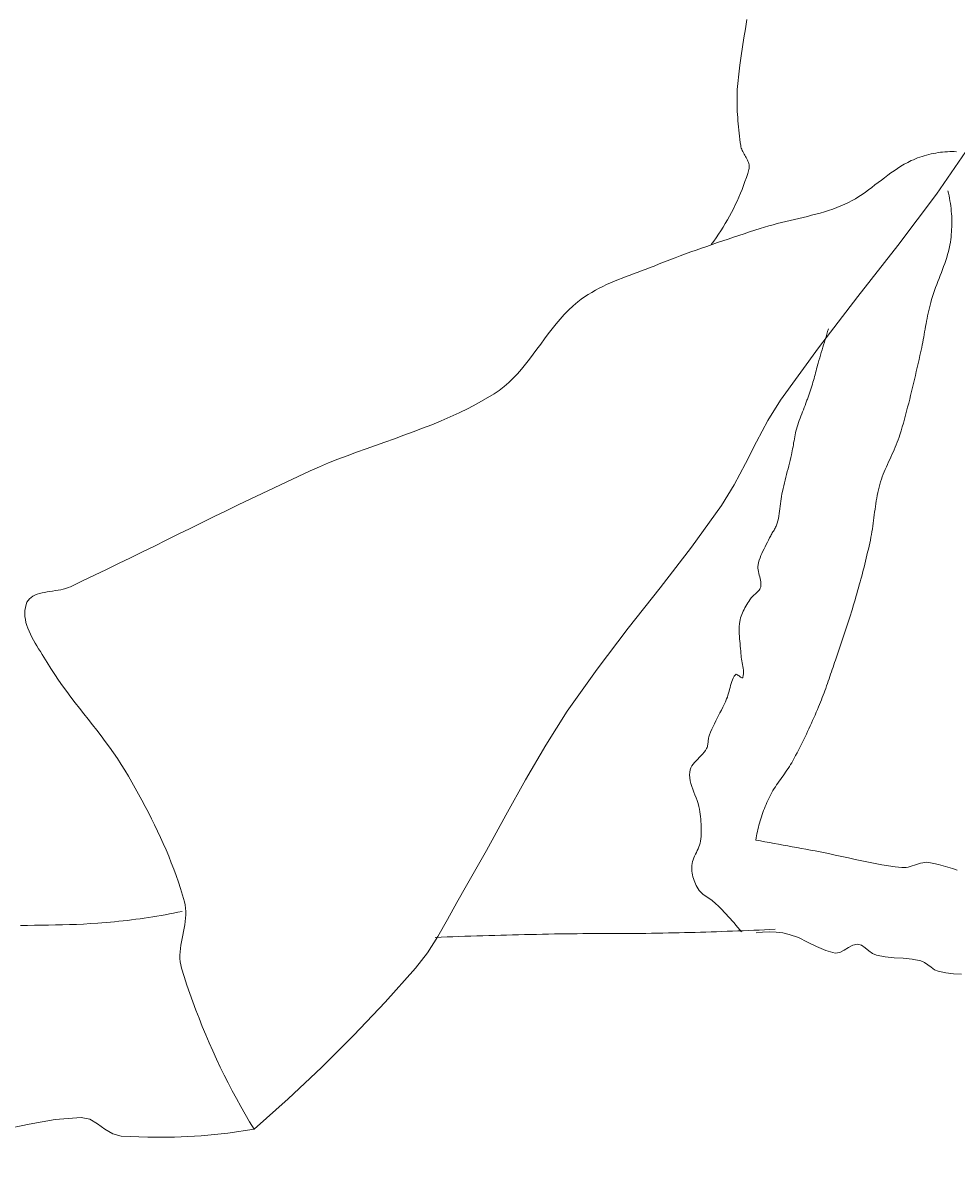
# Model space of a CAD drawing. Units: inches. Extents: x -15 to 423, y -713 to 71.
# Tile 20 of 24: x 311 to 340, y -173 to -137. Entities that reach past the tile are written whole.
import ezdxf

# ---------------------------------------------------------------- set-up
doc = ezdxf.new("R2010")
doc.units = ezdxf.units.IN
doc.header["$MEASUREMENT"] = 0
doc.layers.add('A-ANNO-DIMS', color=2, linetype='Continuous', lineweight=18)
doc.layers.add('A-FURN', color=9, linetype='Continuous', lineweight=13)
doc.styles.get("Standard").update_dxf_attribs({"font": 'arial.ttf'})
doc.dimstyles.get("Standard").update_dxf_attribs({"dimtxt": 0.18, "dimasz": 0.18, "dimexe": 0.18, "dimexo": 0.0625, "dimgap": 0.09, "dimtad": 0, "dimtih": 1, "dimtoh": 1, "dimdec": 0, "dimzin": 0, "dimdsep": 46, "dimlunit": 3, "dimtxsty": 'Standard', "dimcen": 0.09, "dimadec": 0, "dimazin": 0, "dimtfac": 1, "dimtdec": 0, "dimtofl": 0, "dimtmove": 0, "dimatfit": 3, "dimfxl": 1, "dimtolj": 1, "dimtzin": 0, "dimarcsym": 0})

# ---------------------------------------------------------------- blocks, each defined once
blk = doc.blocks.new('BED-DOUBLE')
for p, q in [((72.054, 34.699), (72.006, 34.418)), ((72.006, 34.418), (71.96, 34.136)), ((71.96, 34.136), (71.916, 33.855)), ((71.916, 33.855), (71.875, 33.573)), ((71.837, 33.29), (71.802, 33.008)), ((71.875, 33.573), (71.837, 33.29)), ((71.802, 33.008), (71.771, 32.725)), ((71.762, 32.629), (71.755, 32.532)), ((71.771, 32.725), (71.762, 32.629)), ((71.747, 32.34), (71.746, 32.243)), ((71.746, 32.243), (71.746, 32.147)), ((71.75, 32.436), (71.747, 32.34)), ((71.755, 32.532), (71.75, 32.436)), ((71.746, 32.147), (71.748, 32.05)), ((71.748, 32.05), (71.751, 31.954)), ((71.751, 31.954), (71.755, 31.857)), ((71.755, 31.857), (71.76, 31.761)), ((71.76, 31.761), (71.767, 31.664)), ((71.767, 31.664), (71.775, 31.568)), ((71.775, 31.568), (71.783, 31.471)), ((71.783, 31.471), (71.792, 31.375)), ((71.792, 31.375), (71.802, 31.278)), ((71.802, 31.278), (71.813, 31.182)), ((71.813, 31.182), (71.824, 31.086)), ((71.824, 31.086), (71.836, 30.99)), ((71.836, 30.99), (71.848, 30.894)), ((71.848, 30.894), (71.86, 30.798)), ((71.86, 30.798), (71.867, 30.759)), ((71.867, 30.759), (71.877, 30.721)), ((79.064, 30.944), (77.93, 29.295)), ((71.877, 30.721), (71.891, 30.683)), ((71.891, 30.683), (71.906, 30.645)), ((71.906, 30.645), (71.924, 30.608)), ((71.924, 30.608), (71.944, 30.57)), ((71.944, 30.57), (71.964, 30.533)), ((71.964, 30.533), (71.985, 30.496)), ((71.985, 30.496), (72.007, 30.459)), ((72.007, 30.459), (72.027, 30.423)), ((72.027, 30.423), (72.048, 30.386)), ((77.276, 30.387), (77.343, 30.414)), ((77.343, 30.414), (77.411, 30.439)), ((77.411, 30.439), (77.48, 30.462)), ((77.48, 30.462), (77.549, 30.483)), ((77.549, 30.483), (77.619, 30.503)), ((77.619, 30.503), (77.689, 30.522)), ((77.689, 30.522), (77.76, 30.538)), ((77.76, 30.538), (77.831, 30.553)), ((77.831, 30.553), (77.902, 30.566)), ((77.902, 30.566), (77.974, 30.578)), ((77.974, 30.578), (78.046, 30.588)), ((78.046, 30.588), (78.118, 30.595)), ((78.118, 30.595), (78.19, 30.602)), ((78.19, 30.602), (78.263, 30.606)), ((78.263, 30.606), (78.335, 30.609)), ((78.335, 30.609), (78.407, 30.61)), ((78.407, 30.61), (78.479, 30.609)), ((78.479, 30.609), (78.551, 30.606)), ((72.048, 30.386), (72.066, 30.349)), ((72.066, 30.349), (72.083, 30.313)), ((72.114, 30.054), (72.076, 29.929)), ((72.083, 30.313), (72.098, 30.276)), ((72.098, 30.276), (72.11, 30.239)), ((72.11, 30.239), (72.119, 30.203)), ((72.122, 30.091), (72.114, 30.054)), ((72.119, 30.203), (72.125, 30.166)), ((72.126, 30.129), (72.122, 30.091)), ((72.125, 30.166), (72.126, 30.129)), ((76.616, 30.019), (76.718, 30.088)), ((76.718, 30.088), (76.822, 30.154)), ((76.822, 30.154), (76.927, 30.216)), ((76.927, 30.216), (77.035, 30.275)), ((77.035, 30.275), (77.145, 30.33)), ((77.145, 30.33), (77.21, 30.359)), ((77.21, 30.359), (77.276, 30.387)), ((71.993, 29.682), (71.948, 29.56)), ((72.035, 29.805), (71.993, 29.682)), ((72.076, 29.929), (72.035, 29.805)), ((76.12, 29.65), (76.218, 29.726)), ((76.218, 29.726), (76.316, 29.801)), ((76.316, 29.801), (76.415, 29.875)), ((76.415, 29.875), (76.515, 29.948)), ((76.515, 29.948), (76.616, 30.019)), ((71.901, 29.438), (71.852, 29.317)), ((71.948, 29.56), (71.901, 29.438)), ((75.622, 29.284), (75.724, 29.354)), ((75.724, 29.354), (75.824, 29.426)), ((75.824, 29.426), (75.923, 29.5)), ((75.923, 29.5), (76.021, 29.575)), ((76.021, 29.575), (76.12, 29.65)), ((78.278, 29.398), (78.297, 29.321)), ((71.747, 29.077), (71.691, 28.958)), ((71.8, 29.196), (71.747, 29.077)), ((71.852, 29.317), (71.8, 29.196)), ((74.965, 28.926), (75.09, 28.98)), ((75.09, 28.98), (75.201, 29.033)), ((75.201, 29.033), (75.31, 29.09)), ((75.31, 29.09), (75.416, 29.151)), ((75.416, 29.151), (75.52, 29.216)), ((75.52, 29.216), (75.622, 29.284)), ((77.93, 29.295), (76.727, 27.695)), ((78.297, 29.321), (78.315, 29.242)), ((78.315, 29.242), (78.33, 29.164)), ((78.33, 29.164), (78.345, 29.085)), ((78.345, 29.085), (78.357, 29.005)), ((78.357, 29.005), (78.368, 28.925)), ((71.512, 28.609), (71.448, 28.495)), ((71.574, 28.724), (71.512, 28.609)), ((71.634, 28.841), (71.574, 28.724)), ((71.691, 28.958), (71.634, 28.841)), ((73.926, 28.602), (74.058, 28.635)), ((74.058, 28.635), (74.19, 28.67)), ((74.19, 28.67), (74.322, 28.706)), ((74.322, 28.706), (74.452, 28.745)), ((74.452, 28.745), (74.582, 28.786)), ((74.582, 28.786), (74.711, 28.829)), ((74.711, 28.829), (74.839, 28.876)), ((74.839, 28.876), (74.965, 28.926)), ((78.368, 28.925), (78.378, 28.845)), ((78.378, 28.845), (78.386, 28.765)), ((78.386, 28.765), (78.392, 28.685)), ((78.392, 28.685), (78.397, 28.604)), ((71.315, 28.27), (71.246, 28.159)), ((71.383, 28.381), (71.315, 28.27)), ((71.448, 28.495), (71.383, 28.381)), ((72.468, 28.228), (72.598, 28.269)), ((72.598, 28.269), (72.729, 28.307)), ((72.729, 28.307), (72.861, 28.343)), ((72.861, 28.343), (72.993, 28.378)), ((72.993, 28.378), (73.126, 28.411)), ((73.126, 28.411), (73.259, 28.443)), ((73.259, 28.443), (73.392, 28.475)), ((73.392, 28.475), (73.526, 28.506)), ((73.526, 28.506), (73.659, 28.538)), ((73.659, 28.538), (73.793, 28.569)), ((73.793, 28.569), (73.926, 28.602)), ((78.4, 28.282), (78.396, 28.201)), ((78.397, 28.604), (78.4, 28.524)), ((78.4, 28.524), (78.401, 28.443)), ((78.401, 28.362), (78.4, 28.282)), ((78.401, 28.443), (78.401, 28.362)), ((71.101, 27.942), (71.026, 27.835)), ((71.175, 28.05), (71.101, 27.942)), ((71.246, 28.159), (71.175, 28.05)), ((71.307, 27.845), (71.472, 27.9)), ((71.472, 27.9), (71.638, 27.956)), ((71.638, 27.956), (71.804, 28.011)), ((71.804, 28.011), (71.97, 28.065)), ((71.97, 28.065), (72.136, 28.12)), ((72.136, 28.12), (72.302, 28.174)), ((72.302, 28.174), (72.468, 28.228)), ((78.377, 27.961), (78.367, 27.882)), ((78.385, 28.041), (78.377, 27.961)), ((78.392, 28.121), (78.385, 28.041)), ((78.396, 28.201), (78.392, 28.121)), ((70.317, 27.499), (70.481, 27.558)), ((70.481, 27.558), (70.646, 27.616)), ((70.646, 27.616), (70.811, 27.674)), ((70.811, 27.674), (70.976, 27.732)), ((71.026, 27.835), (70.95, 27.73)), ((70.976, 27.732), (71.141, 27.788)), ((71.141, 27.788), (71.307, 27.845)), ((76.727, 27.695), (75.494, 26.115)), ((78.319, 27.61), (78.296, 27.515)), ((78.339, 27.706), (78.319, 27.61)), ((78.356, 27.803), (78.339, 27.706)), ((78.367, 27.882), (78.356, 27.803)), ((69.337, 27.129), (69.499, 27.193)), ((69.499, 27.193), (69.662, 27.255)), ((69.662, 27.255), (69.826, 27.318)), ((69.826, 27.318), (69.989, 27.379)), ((69.989, 27.379), (70.153, 27.439)), ((70.153, 27.439), (70.317, 27.499)), ((78.213, 27.233), (78.181, 27.139)), ((78.243, 27.326), (78.213, 27.233)), ((78.271, 27.42), (78.243, 27.326)), ((78.296, 27.515), (78.271, 27.42)), ((68.438, 26.784), (68.561, 26.831)), ((68.561, 26.831), (68.685, 26.877)), ((68.685, 26.877), (68.808, 26.923)), ((68.808, 26.923), (68.931, 26.969)), ((68.931, 26.969), (69.053, 27.016)), ((69.053, 27.016), (69.175, 27.064)), ((69.175, 27.064), (69.337, 27.129)), ((78.078, 26.862), (78.042, 26.77)), ((78.113, 26.954), (78.078, 26.862)), ((78.147, 27.047), (78.113, 26.954)), ((78.181, 27.139), (78.147, 27.047)), ((67.589, 26.431), (67.707, 26.487)), ((67.707, 26.487), (67.826, 26.54)), ((67.826, 26.54), (67.947, 26.592)), ((67.947, 26.592), (68.069, 26.642)), ((68.069, 26.642), (68.191, 26.69)), ((68.191, 26.69), (68.314, 26.738)), ((68.314, 26.738), (68.438, 26.784)), ((77.934, 26.493), (77.9, 26.401)), ((77.97, 26.585), (77.934, 26.493)), ((78.006, 26.678), (77.97, 26.585)), ((78.042, 26.77), (78.006, 26.678)), ((66.919, 26.035), (67.025, 26.11)), ((67.025, 26.11), (67.133, 26.181)), ((67.133, 26.181), (67.244, 26.248)), ((67.244, 26.248), (67.357, 26.312)), ((67.357, 26.312), (67.472, 26.373)), ((67.472, 26.373), (67.589, 26.431)), ((75.494, 26.115), (74.271, 24.528)), ((77.802, 26.121), (77.774, 26.027)), ((77.833, 26.215), (77.802, 26.121)), ((77.866, 26.308), (77.833, 26.215)), ((77.9, 26.401), (77.866, 26.308)), ((66.528, 25.699), (66.668, 25.831)), ((66.668, 25.831), (66.815, 25.956)), ((66.815, 25.956), (66.919, 26.035)), ((77.706, 25.77), (77.687, 25.688)), ((77.726, 25.851), (77.706, 25.77)), ((77.747, 25.932), (77.726, 25.851)), ((77.774, 26.027), (77.747, 25.932)), ((66.139, 25.268), (66.264, 25.417)), ((66.264, 25.417), (66.394, 25.561)), ((66.394, 25.561), (66.528, 25.699)), ((77.636, 25.442), (77.62, 25.36)), ((77.652, 25.524), (77.636, 25.442)), ((77.669, 25.606), (77.652, 25.524)), ((77.687, 25.688), (77.669, 25.606)), ((65.898, 24.96), (66.017, 25.115)), ((66.017, 25.115), (66.139, 25.268)), ((74.553, 25.034), (74.528, 24.953)), ((74.579, 25.115), (74.553, 25.034)), ((77.574, 25.112), (77.56, 25.029)), ((77.589, 25.195), (77.574, 25.112)), ((77.604, 25.277), (77.589, 25.195)), ((77.62, 25.36), (77.604, 25.277)), ((65.664, 24.644), (65.781, 24.803)), ((65.781, 24.803), (65.898, 24.96)), ((74.454, 24.708), (74.43, 24.626)), ((74.479, 24.79), (74.454, 24.708)), ((74.504, 24.871), (74.479, 24.79)), ((74.528, 24.953), (74.504, 24.871)), ((77.5, 24.699), (77.485, 24.617)), ((77.516, 24.782), (77.5, 24.699)), ((77.53, 24.864), (77.516, 24.782)), ((77.545, 24.947), (77.53, 24.864)), ((77.56, 25.029), (77.545, 24.947)), ((65.313, 24.173), (65.432, 24.329)), ((65.432, 24.329), (65.548, 24.486)), ((65.548, 24.486), (65.664, 24.644)), ((74.271, 24.528), (73.096, 22.907)), ((74.357, 24.381), (74.333, 24.3)), ((74.381, 24.463), (74.357, 24.381)), ((74.405, 24.545), (74.381, 24.463)), ((74.43, 24.626), (74.405, 24.545)), ((77.434, 24.37), (77.415, 24.288)), ((77.452, 24.452), (77.434, 24.37)), ((77.468, 24.534), (77.452, 24.452)), ((77.485, 24.617), (77.468, 24.534)), ((65.07, 23.871), (65.193, 24.02)), ((65.193, 24.02), (65.313, 24.173)), ((74.244, 23.995), (74.228, 23.936)), ((74.261, 24.054), (74.244, 23.995)), ((74.285, 24.136), (74.261, 24.054)), ((74.309, 24.218), (74.285, 24.136)), ((74.333, 24.3), (74.309, 24.218)), ((77.358, 24.042), (77.33, 23.918)), ((77.387, 24.165), (77.358, 24.042)), ((77.415, 24.288), (77.387, 24.165)), ((64.81, 23.587), (64.942, 23.726)), ((64.942, 23.726), (65.07, 23.871)), ((74.148, 23.638), (74.132, 23.578)), ((74.164, 23.697), (74.148, 23.638)), ((74.18, 23.757), (74.164, 23.697)), ((74.196, 23.817), (74.18, 23.757)), ((74.212, 23.876), (74.196, 23.817)), ((74.228, 23.936), (74.212, 23.876)), ((77.272, 23.672), (77.244, 23.548)), ((77.301, 23.795), (77.272, 23.672)), ((77.33, 23.918), (77.301, 23.795)), ((64.378, 23.211), (64.529, 23.329)), ((64.529, 23.329), (64.673, 23.454)), ((64.673, 23.454), (64.81, 23.587)), ((74.038, 23.25), (74.028, 23.219)), ((74.048, 23.282), (74.038, 23.25)), ((74.066, 23.341), (74.048, 23.282)), ((74.083, 23.4), (74.066, 23.341)), ((74.1, 23.46), (74.083, 23.4)), ((74.116, 23.519), (74.1, 23.46)), ((74.132, 23.578), (74.116, 23.519)), ((77.185, 23.302), (77.156, 23.179)), ((77.215, 23.425), (77.185, 23.302)), ((77.244, 23.548), (77.215, 23.425)), ((63.688, 22.792), (63.956, 22.943)), ((63.956, 22.943), (64.219, 23.104)), ((64.219, 23.104), (64.378, 23.211)), ((73.096, 22.907), (72.702, 22.273)), ((73.913, 22.909), (73.902, 22.877)), ((73.925, 22.94), (73.913, 22.909)), ((73.937, 22.971), (73.925, 22.94)), ((73.948, 23.002), (73.937, 22.971)), ((73.96, 23.032), (73.948, 23.002)), ((73.972, 23.063), (73.96, 23.032)), ((73.983, 23.094), (73.972, 23.063)), ((73.995, 23.125), (73.983, 23.094)), ((74.006, 23.157), (73.995, 23.125)), ((74.017, 23.188), (74.006, 23.157)), ((74.028, 23.219), (74.017, 23.188)), ((77.096, 22.933), (77.065, 22.81)), ((77.126, 23.056), (77.096, 22.933)), ((77.156, 23.179), (77.126, 23.056)), ((63.139, 22.515), (63.415, 22.65)), ((63.415, 22.65), (63.688, 22.792)), ((73.776, 22.546), (73.751, 22.48)), ((73.802, 22.612), (73.776, 22.546)), ((73.827, 22.678), (73.802, 22.612)), ((73.853, 22.744), (73.827, 22.678)), ((73.878, 22.811), (73.853, 22.744)), ((73.902, 22.877), (73.878, 22.811)), ((77.001, 22.565), (76.968, 22.443)), ((77.033, 22.688), (77.001, 22.565)), ((77.065, 22.81), (77.033, 22.688)), ((62.291, 22.147), (62.576, 22.264)), ((62.576, 22.264), (62.859, 22.386)), ((62.859, 22.386), (63.139, 22.515)), ((72.702, 22.273), (72.35, 21.612)), ((73.653, 22.213), (73.631, 22.146)), ((73.676, 22.28), (73.653, 22.213)), ((73.701, 22.347), (73.676, 22.28)), ((73.725, 22.413), (73.701, 22.347)), ((73.751, 22.48), (73.725, 22.413)), ((76.9, 22.199), (76.865, 22.078)), ((76.935, 22.321), (76.9, 22.199)), ((76.968, 22.443), (76.935, 22.321)), ((61.13, 21.712), (61.422, 21.817)), ((61.422, 21.817), (61.713, 21.924)), ((61.713, 21.924), (62.003, 22.034)), ((62.003, 22.034), (62.291, 22.147)), ((73.546, 21.829), (73.534, 21.768)), ((73.559, 21.89), (73.546, 21.829)), ((73.573, 21.95), (73.559, 21.89)), ((73.59, 22.01), (73.573, 21.95)), ((73.609, 22.079), (73.59, 22.01)), ((73.631, 22.146), (73.609, 22.079)), ((76.792, 21.835), (76.766, 21.756)), ((76.829, 21.956), (76.792, 21.835)), ((76.865, 22.078), (76.829, 21.956)), ((60.252, 21.4), (60.545, 21.504)), ((60.545, 21.504), (60.838, 21.608)), ((60.838, 21.608), (61.13, 21.712)), ((72.35, 21.612), (72.012, 20.943)), ((73.481, 21.462), (73.47, 21.4)), ((73.491, 21.523), (73.481, 21.462)), ((73.501, 21.585), (73.491, 21.523)), ((73.512, 21.646), (73.501, 21.585)), ((73.522, 21.707), (73.512, 21.646)), ((73.534, 21.768), (73.522, 21.707)), ((76.679, 21.524), (76.647, 21.447)), ((76.709, 21.601), (76.679, 21.524)), ((76.739, 21.678), (76.709, 21.601)), ((76.766, 21.756), (76.739, 21.678)), ((59.38, 21.075), (59.67, 21.186)), ((59.67, 21.186), (59.96, 21.294)), ((59.96, 21.294), (60.252, 21.4)), ((73.414, 21.13), (73.393, 21.042)), ((73.434, 21.217), (73.414, 21.13)), ((73.447, 21.278), (73.434, 21.217)), ((73.459, 21.339), (73.447, 21.278)), ((73.47, 21.4), (73.459, 21.339)), ((76.511, 21.143), (76.476, 21.067)), ((76.546, 21.219), (76.511, 21.143)), ((76.58, 21.294), (76.546, 21.219)), ((76.614, 21.371), (76.58, 21.294)), ((76.647, 21.447), (76.614, 21.371)), ((58.525, 20.716), (58.808, 20.841)), ((58.808, 20.841), (59.093, 20.96)), ((59.093, 20.96), (59.38, 21.075)), ((72.012, 20.943), (71.661, 20.282)), ((73.326, 20.779), (73.303, 20.692)), ((73.348, 20.867), (73.326, 20.779)), ((73.371, 20.954), (73.348, 20.867)), ((73.393, 21.042), (73.371, 20.954)), ((76.34, 20.763), (76.308, 20.687)), ((76.373, 20.84), (76.34, 20.763)), ((76.407, 20.916), (76.373, 20.84)), ((76.441, 20.991), (76.407, 20.916)), ((76.476, 21.067), (76.441, 20.991)), ((57.776, 20.37), (58.15, 20.544)), ((58.15, 20.544), (58.525, 20.716)), ((73.235, 20.429), (73.214, 20.342)), ((73.257, 20.517), (73.235, 20.429)), ((73.28, 20.604), (73.257, 20.517)), ((73.303, 20.692), (73.28, 20.604)), ((76.221, 20.454), (76.195, 20.375)), ((76.248, 20.532), (76.221, 20.454)), ((76.278, 20.61), (76.248, 20.532)), ((76.308, 20.687), (76.278, 20.61)), ((57.029, 20.017), (57.402, 20.194)), ((57.402, 20.194), (57.776, 20.37)), ((71.661, 20.282), (71.268, 19.647)), ((73.154, 20.078), (73.139, 20.002)), ((73.173, 20.166), (73.154, 20.078)), ((73.193, 20.254), (73.173, 20.166)), ((73.214, 20.342), (73.193, 20.254)), ((76.109, 20.041), (76.092, 19.956)), ((76.128, 20.127), (76.109, 20.041)), ((76.149, 20.211), (76.128, 20.127)), ((76.171, 20.296), (76.149, 20.211)), ((76.195, 20.375), (76.171, 20.296)), ((56.286, 19.659), (56.657, 19.838)), ((56.657, 19.838), (57.029, 20.017)), ((73.095, 19.697), (73.085, 19.621)), ((73.104, 19.774), (73.095, 19.697)), ((73.115, 19.85), (73.104, 19.774)), ((73.126, 19.926), (73.115, 19.85)), ((73.139, 20.002), (73.126, 19.926)), ((76.048, 19.698), (76.035, 19.611)), ((76.062, 19.784), (76.048, 19.698)), ((76.076, 19.87), (76.062, 19.784)), ((76.092, 19.956), (76.076, 19.87)), ((55.544, 19.297), (55.915, 19.478)), ((55.915, 19.478), (56.286, 19.659)), ((71.268, 19.647), (70.336, 18.355)), ((73.042, 19.316), (73.028, 19.24)), ((73.054, 19.392), (73.042, 19.316)), ((73.065, 19.468), (73.054, 19.392)), ((73.076, 19.544), (73.065, 19.468)), ((73.085, 19.621), (73.076, 19.544)), ((75.999, 19.351), (75.988, 19.264)), ((76.011, 19.438), (75.999, 19.351)), ((76.023, 19.524), (76.011, 19.438)), ((76.035, 19.611), (76.023, 19.524)), ((54.803, 18.932), (55.173, 19.115)), ((55.173, 19.115), (55.544, 19.297)), ((72.943, 18.968), (72.927, 18.938)), ((72.958, 18.997), (72.943, 18.968)), ((72.972, 19.028), (72.958, 18.997)), ((72.984, 19.059), (72.972, 19.028)), ((72.994, 19.09), (72.984, 19.059)), ((73.012, 19.165), (72.994, 19.09)), ((73.028, 19.24), (73.012, 19.165)), ((75.952, 19.004), (75.939, 18.917)), ((75.965, 19.09), (75.952, 19.004)), ((75.976, 19.177), (75.965, 19.09)), ((75.988, 19.264), (75.976, 19.177)), ((54.063, 18.567), (54.433, 18.75)), ((54.433, 18.75), (54.803, 18.932)), ((72.757, 18.638), (72.723, 18.57)), ((72.79, 18.707), (72.757, 18.638)), ((72.805, 18.737), (72.79, 18.707)), ((72.821, 18.766), (72.805, 18.737)), ((72.838, 18.795), (72.821, 18.766)), ((72.856, 18.824), (72.838, 18.795)), ((72.874, 18.852), (72.856, 18.824)), ((72.892, 18.881), (72.874, 18.852)), ((72.91, 18.91), (72.892, 18.881)), ((72.927, 18.938), (72.91, 18.91)), ((75.894, 18.659), (75.877, 18.573)), ((75.911, 18.745), (75.894, 18.659)), ((75.925, 18.831), (75.911, 18.745)), ((75.939, 18.917), (75.925, 18.831)), ((53.322, 18.202), (53.692, 18.384)), ((53.692, 18.384), (54.063, 18.567)), ((70.336, 18.355), (69.362, 17.092)), ((72.583, 18.298), (72.55, 18.229)), ((72.618, 18.366), (72.583, 18.298)), ((72.653, 18.434), (72.618, 18.366)), ((72.688, 18.502), (72.653, 18.434)), ((72.723, 18.57), (72.688, 18.502)), ((75.815, 18.293), (75.793, 18.2)), ((75.836, 18.386), (75.815, 18.293)), ((75.857, 18.48), (75.836, 18.386)), ((75.877, 18.573), (75.857, 18.48)), ((52.58, 17.84), (52.951, 18.021)), ((52.951, 18.021), (53.322, 18.202)), ((72.436, 17.949), (72.415, 17.876)), ((72.461, 18.02), (72.436, 17.949)), ((72.488, 18.091), (72.461, 18.02)), ((72.518, 18.16), (72.488, 18.091)), ((72.55, 18.229), (72.518, 18.16)), ((75.727, 17.92), (75.704, 17.827)), ((75.749, 18.013), (75.727, 17.92)), ((75.772, 18.106), (75.749, 18.013)), ((75.793, 18.2), (75.772, 18.106)), ((51.837, 17.48), (52.209, 17.659)), ((52.209, 17.659), (52.58, 17.84)), ((72.399, 17.803), (72.392, 17.751)), ((72.392, 17.751), (72.392, 17.698)), ((72.392, 17.698), (72.398, 17.646)), ((72.398, 17.646), (72.408, 17.593)), ((72.415, 17.876), (72.399, 17.803)), ((72.408, 17.593), (72.421, 17.54)), ((72.421, 17.54), (72.435, 17.487)), ((75.633, 17.549), (75.609, 17.457)), ((75.657, 17.642), (75.633, 17.549)), ((75.681, 17.735), (75.657, 17.642)), ((75.704, 17.827), (75.681, 17.735)), ((51.091, 17.126), (51.465, 17.303)), ((51.465, 17.303), (51.837, 17.48)), ((72.435, 17.487), (72.45, 17.434)), ((72.45, 17.434), (72.464, 17.382)), ((72.464, 17.382), (72.476, 17.329)), ((72.476, 17.329), (72.485, 17.276)), ((72.488, 17.172), (72.479, 17.121)), ((72.485, 17.276), (72.489, 17.224)), ((72.489, 17.224), (72.488, 17.172)), ((75.534, 17.179), (75.509, 17.087)), ((75.559, 17.272), (75.534, 17.179)), ((75.584, 17.364), (75.559, 17.272)), ((75.609, 17.457), (75.584, 17.364)), ((49.873, 16.795), (49.93, 16.832)), ((49.93, 16.832), (49.993, 16.864)), ((49.993, 16.864), (50.062, 16.891)), ((50.062, 16.891), (50.135, 16.914)), ((50.135, 16.914), (50.211, 16.933)), ((50.211, 16.933), (50.291, 16.95)), ((50.291, 16.95), (50.373, 16.965)), ((50.373, 16.965), (50.456, 16.978)), ((50.456, 16.978), (50.541, 16.991)), ((50.541, 16.991), (50.625, 17.004)), ((50.625, 17.004), (50.709, 17.018)), ((50.709, 17.018), (50.791, 17.034)), ((50.791, 17.034), (50.871, 17.052)), ((50.871, 17.052), (50.948, 17.073)), ((50.948, 17.073), (51.022, 17.097)), ((51.022, 17.097), (51.091, 17.126)), ((69.362, 17.092), (68.377, 15.838)), ((72.217, 16.815), (72.188, 16.785)), ((72.248, 16.844), (72.217, 16.815)), ((72.28, 16.872), (72.248, 16.844)), ((72.312, 16.899), (72.28, 16.872)), ((72.344, 16.927), (72.312, 16.899)), ((72.374, 16.955), (72.344, 16.927)), ((72.402, 16.984), (72.374, 16.955)), ((72.428, 17.015), (72.402, 16.984)), ((72.45, 17.048), (72.428, 17.015)), ((72.467, 17.083), (72.45, 17.048)), ((72.479, 17.121), (72.467, 17.083)), ((75.431, 16.811), (75.404, 16.719)), ((75.457, 16.903), (75.431, 16.811)), ((75.483, 16.995), (75.457, 16.903)), ((75.509, 17.087), (75.483, 16.995)), ((49.682, 16.392), (49.695, 16.485)), ((49.695, 16.485), (49.718, 16.577)), ((49.718, 16.577), (49.744, 16.643)), ((49.744, 16.643), (49.779, 16.701)), ((49.779, 16.701), (49.822, 16.751)), ((49.822, 16.751), (49.873, 16.795)), ((71.993, 16.473), (71.965, 16.422)), ((72.021, 16.523), (71.993, 16.473)), ((72.05, 16.573), (72.021, 16.523)), ((72.08, 16.623), (72.05, 16.573)), ((72.11, 16.672), (72.08, 16.623)), ((72.139, 16.721), (72.11, 16.672)), ((72.162, 16.754), (72.139, 16.721)), ((72.188, 16.785), (72.162, 16.754)), ((75.348, 16.53), (75.32, 16.436)), ((75.376, 16.625), (75.348, 16.53)), ((75.404, 16.719), (75.376, 16.625)), ((49.678, 16.3), (49.682, 16.392)), ((49.683, 16.207), (49.678, 16.3)), ((49.695, 16.114), (49.683, 16.207)), ((49.715, 16.021), (49.695, 16.114)), ((71.842, 16.104), (71.831, 16.048)), ((71.856, 16.159), (71.842, 16.104)), ((71.874, 16.213), (71.856, 16.159)), ((71.893, 16.266), (71.874, 16.213)), ((71.915, 16.319), (71.893, 16.266)), ((71.94, 16.371), (71.915, 16.319)), ((71.965, 16.422), (71.94, 16.371)), ((75.232, 16.155), (75.202, 16.061)), ((75.262, 16.248), (75.232, 16.155)), ((75.291, 16.342), (75.262, 16.248)), ((75.32, 16.436), (75.291, 16.342)), ((49.741, 15.928), (49.715, 16.021)), ((49.773, 15.836), (49.741, 15.928)), ((49.811, 15.743), (49.773, 15.836)), ((49.853, 15.651), (49.811, 15.743)), ((68.377, 15.838), (67.408, 14.572)), ((71.815, 15.897), (71.812, 15.821)), ((71.812, 15.821), (71.812, 15.745)), ((71.812, 15.745), (71.814, 15.668)), ((71.821, 15.972), (71.815, 15.897)), ((71.831, 16.048), (71.821, 15.972)), ((75.11, 15.78), (75.079, 15.687)), ((75.141, 15.874), (75.11, 15.78)), ((75.172, 15.967), (75.141, 15.874)), ((75.202, 16.061), (75.172, 15.967)), ((49.898, 15.56), (49.853, 15.651)), ((49.947, 15.469), (49.898, 15.56)), ((49.999, 15.379), (49.947, 15.469)), ((50.052, 15.289), (49.999, 15.379)), ((71.814, 15.668), (71.819, 15.592)), ((71.819, 15.592), (71.825, 15.515)), ((71.825, 15.515), (71.832, 15.439)), ((71.832, 15.439), (71.839, 15.362)), ((74.985, 15.407), (74.954, 15.314)), ((75.017, 15.5), (74.985, 15.407)), ((75.048, 15.594), (75.017, 15.5)), ((75.079, 15.687), (75.048, 15.594)), ((50.106, 15.2), (50.052, 15.289)), ((50.161, 15.113), (50.106, 15.2)), ((50.216, 15.026), (50.161, 15.113)), ((50.27, 14.94), (50.216, 15.026)), ((71.839, 15.362), (71.847, 15.285)), ((71.847, 15.285), (71.854, 15.209)), ((71.854, 15.209), (71.86, 15.132)), ((71.86, 15.132), (71.865, 15.056)), ((71.865, 15.056), (71.87, 14.999)), ((74.859, 15.035), (74.827, 14.942)), ((74.89, 15.128), (74.859, 15.035)), ((74.922, 15.221), (74.89, 15.128)), ((74.954, 15.314), (74.922, 15.221)), ((50.323, 14.856), (50.27, 14.94)), ((50.373, 14.773), (50.323, 14.856)), ((50.486, 14.588), (50.373, 14.773)), ((71.87, 14.999), (71.877, 14.942)), ((71.877, 14.942), (71.887, 14.884)), ((71.887, 14.884), (71.897, 14.827)), ((71.897, 14.827), (71.908, 14.769)), ((71.908, 14.769), (71.919, 14.712)), ((71.919, 14.712), (71.928, 14.654)), ((74.746, 14.703), (74.721, 14.63)), ((74.77, 14.776), (74.746, 14.703)), ((74.795, 14.849), (74.77, 14.776)), ((74.827, 14.942), (74.795, 14.849)), ((50.604, 14.407), (50.486, 14.588)), ((50.725, 14.228), (50.604, 14.407)), ((67.408, 14.572), (66.487, 13.273)), ((71.66, 14.349), (71.63, 14.296)), ((71.694, 14.399), (71.66, 14.349)), ((71.707, 14.41), (71.694, 14.399)), ((71.724, 14.411), (71.707, 14.41)), ((71.743, 14.405), (71.724, 14.411)), ((71.764, 14.394), (71.743, 14.405)), ((71.786, 14.379), (71.764, 14.394)), ((71.809, 14.361), (71.786, 14.379)), ((71.831, 14.344), (71.809, 14.361)), ((71.853, 14.327), (71.831, 14.344)), ((71.873, 14.313), (71.853, 14.327)), ((71.891, 14.303), (71.873, 14.313)), ((71.925, 14.316), (71.918, 14.303)), ((71.937, 14.371), (71.925, 14.316)), ((71.928, 14.654), (71.936, 14.597)), ((71.936, 14.597), (71.942, 14.54)), ((71.943, 14.427), (71.937, 14.371)), ((71.942, 14.54), (71.944, 14.484)), ((71.944, 14.484), (71.943, 14.427)), ((74.623, 14.339), (74.598, 14.266)), ((74.647, 14.412), (74.623, 14.339)), ((74.672, 14.485), (74.647, 14.412)), ((74.697, 14.557), (74.672, 14.485)), ((74.721, 14.63), (74.697, 14.557)), ((50.85, 14.051), (50.725, 14.228)), ((50.978, 13.876), (50.85, 14.051)), ((71.53, 14.005), (71.515, 13.945)), ((71.546, 14.066), (71.53, 14.005)), ((71.563, 14.125), (71.546, 14.066)), ((71.583, 14.184), (71.563, 14.125)), ((71.605, 14.241), (71.583, 14.184)), ((71.63, 14.296), (71.605, 14.241)), ((71.907, 14.299), (71.891, 14.303)), ((71.918, 14.303), (71.907, 14.299)), ((74.496, 13.976), (74.47, 13.904)), ((74.522, 14.049), (74.496, 13.976)), ((74.547, 14.121), (74.522, 14.049)), ((74.573, 14.194), (74.547, 14.121)), ((74.598, 14.266), (74.573, 14.194)), ((51.107, 13.702), (50.978, 13.876)), ((51.239, 13.53), (51.107, 13.702)), ((71.423, 13.648), (71.385, 13.561)), ((71.446, 13.705), (71.423, 13.648)), ((71.465, 13.764), (71.446, 13.705)), ((71.483, 13.824), (71.465, 13.764)), ((71.499, 13.884), (71.483, 13.824)), ((71.515, 13.945), (71.499, 13.884)), ((74.361, 13.617), (74.333, 13.546)), ((74.389, 13.688), (74.361, 13.617)), ((74.416, 13.76), (74.389, 13.688)), ((74.443, 13.832), (74.416, 13.76)), ((74.47, 13.904), (74.443, 13.832)), ((51.372, 13.358), (51.239, 13.53)), ((51.506, 13.188), (51.372, 13.358)), ((66.487, 13.273), (65.818, 12.219)), ((71.261, 13.304), (71.218, 13.219)), ((71.303, 13.389), (71.261, 13.304)), ((71.344, 13.475), (71.303, 13.389)), ((71.385, 13.561), (71.344, 13.475)), ((74.201, 13.233), (74.164, 13.148)), ((74.238, 13.318), (74.201, 13.233)), ((74.274, 13.404), (74.238, 13.318)), ((74.304, 13.474), (74.274, 13.404)), ((74.333, 13.546), (74.304, 13.474)), ((51.64, 13.017), (51.506, 13.188)), ((51.775, 12.846), (51.64, 13.017)), ((71.047, 12.88), (71.006, 12.794)), ((71.089, 12.965), (71.047, 12.88)), ((71.132, 13.05), (71.089, 12.965)), ((71.175, 13.135), (71.132, 13.05)), ((71.218, 13.219), (71.175, 13.135)), ((74.051, 12.894), (74.013, 12.81)), ((74.089, 12.979), (74.051, 12.894)), ((74.127, 13.064), (74.089, 12.979)), ((74.164, 13.148), (74.127, 13.064)), ((51.908, 12.675), (51.775, 12.846)), ((52.04, 12.503), (51.908, 12.675)), ((70.891, 12.534), (70.88, 12.502)), ((70.927, 12.621), (70.891, 12.534)), ((70.966, 12.708), (70.927, 12.621)), ((71.006, 12.794), (70.966, 12.708)), ((73.895, 12.558), (73.855, 12.474)), ((73.935, 12.642), (73.895, 12.558)), ((73.974, 12.726), (73.935, 12.642)), ((74.013, 12.81), (73.974, 12.726)), ((52.171, 12.33), (52.04, 12.503)), ((52.299, 12.156), (52.171, 12.33)), ((65.818, 12.219), (65.191, 11.14)), ((70.827, 12.17), (70.816, 12.138)), ((70.836, 12.202), (70.827, 12.17)), ((70.842, 12.235), (70.836, 12.202)), ((70.846, 12.268), (70.842, 12.235)), ((70.85, 12.302), (70.846, 12.268)), ((70.853, 12.336), (70.85, 12.302)), ((70.856, 12.37), (70.853, 12.336)), ((70.86, 12.403), (70.856, 12.37)), ((70.865, 12.437), (70.86, 12.403)), ((70.871, 12.47), (70.865, 12.437)), ((70.88, 12.502), (70.871, 12.47)), ((73.733, 12.225), (73.691, 12.142)), ((73.774, 12.308), (73.733, 12.225)), ((73.815, 12.391), (73.774, 12.308)), ((73.855, 12.474), (73.815, 12.391)), ((52.425, 11.98), (52.299, 12.156)), ((52.548, 11.802), (52.425, 11.98)), ((52.667, 11.621), (52.548, 11.802)), ((70.578, 11.835), (70.527, 11.783)), ((70.629, 11.886), (70.578, 11.835)), ((70.679, 11.939), (70.629, 11.886)), ((70.725, 11.993), (70.679, 11.939)), ((70.767, 12.049), (70.725, 11.993)), ((70.802, 12.108), (70.767, 12.049)), ((70.816, 12.138), (70.802, 12.108)), ((73.519, 11.814), (73.475, 11.732)), ((73.563, 11.895), (73.519, 11.814)), ((73.606, 11.977), (73.563, 11.895)), ((73.649, 12.06), (73.606, 11.977)), ((73.691, 12.142), (73.649, 12.06)), ((52.782, 11.438), (52.667, 11.621)), ((70.293, 11.449), (70.279, 11.383)), ((70.316, 11.511), (70.293, 11.449)), ((70.347, 11.57), (70.316, 11.511)), ((70.385, 11.626), (70.347, 11.57)), ((70.429, 11.68), (70.385, 11.626)), ((70.477, 11.732), (70.429, 11.68)), ((70.527, 11.783), (70.477, 11.732)), ((73.331, 11.495), (73.293, 11.438)), ((73.369, 11.553), (73.331, 11.495)), ((73.406, 11.612), (73.369, 11.553)), ((73.441, 11.672), (73.406, 11.612)), ((73.475, 11.732), (73.441, 11.672)), ((52.892, 11.252), (52.782, 11.438)), ((52.997, 11.067), (52.892, 11.252)), ((65.191, 11.14), (64.585, 10.047)), ((70.279, 11.383), (70.274, 11.292)), ((70.274, 11.292), (70.28, 11.202)), ((70.28, 11.202), (70.294, 11.113)), ((70.294, 11.113), (70.315, 11.025)), ((73.052, 11.097), (73.012, 11.04)), ((73.092, 11.153), (73.052, 11.097)), ((73.132, 11.21), (73.092, 11.153)), ((73.173, 11.267), (73.132, 11.21)), ((73.213, 11.323), (73.173, 11.267)), ((73.253, 11.38), (73.213, 11.323)), ((73.293, 11.438), (73.253, 11.38)), ((53.102, 10.881), (52.997, 11.067)), ((53.205, 10.694), (53.102, 10.881)), ((70.315, 11.025), (70.342, 10.936)), ((70.342, 10.936), (70.373, 10.849)), ((70.373, 10.849), (70.407, 10.761)), ((70.407, 10.761), (70.442, 10.673)), ((72.824, 10.749), (72.79, 10.688)), ((72.859, 10.808), (72.824, 10.749)), ((72.896, 10.867), (72.859, 10.808)), ((72.934, 10.925), (72.896, 10.867)), ((72.972, 10.983), (72.934, 10.925)), ((73.012, 11.04), (72.972, 10.983)), ((53.307, 10.506), (53.205, 10.694)), ((53.407, 10.317), (53.307, 10.506)), ((70.442, 10.673), (70.477, 10.585)), ((70.477, 10.585), (70.51, 10.497)), ((70.51, 10.497), (70.539, 10.408)), ((70.539, 10.408), (70.564, 10.319)), ((72.646, 10.379), (72.62, 10.316)), ((72.672, 10.441), (72.646, 10.379)), ((72.7, 10.503), (72.672, 10.441)), ((72.728, 10.565), (72.7, 10.503)), ((72.758, 10.627), (72.728, 10.565)), ((72.79, 10.688), (72.758, 10.627)), ((53.506, 10.127), (53.407, 10.317)), ((53.603, 9.937), (53.506, 10.127)), ((64.585, 10.047), (63.982, 8.952)), ((70.564, 10.319), (70.582, 10.229)), ((70.582, 10.229), (70.593, 10.153)), ((70.593, 10.153), (70.604, 10.077)), ((70.604, 10.077), (70.613, 10.001)), ((72.526, 10.062), (72.504, 9.997)), ((72.548, 10.126), (72.526, 10.062)), ((72.571, 10.19), (72.548, 10.126)), ((72.595, 10.253), (72.571, 10.19)), ((72.62, 10.316), (72.595, 10.253)), ((53.698, 9.745), (53.603, 9.937)), ((53.791, 9.552), (53.698, 9.745)), ((70.613, 10.001), (70.621, 9.924)), ((70.621, 9.924), (70.628, 9.848)), ((70.628, 9.848), (70.633, 9.771)), ((70.633, 9.771), (70.636, 9.695)), ((70.636, 9.695), (70.638, 9.618)), ((72.41, 9.671), (72.394, 9.605)), ((72.427, 9.736), (72.41, 9.671)), ((72.445, 9.802), (72.427, 9.736)), ((72.464, 9.867), (72.445, 9.802)), ((72.484, 9.932), (72.464, 9.867)), ((72.504, 9.997), (72.484, 9.932)), ((53.881, 9.358), (53.791, 9.552)), ((53.969, 9.163), (53.881, 9.358)), ((70.625, 9.312), (70.616, 9.236)), ((70.631, 9.388), (70.625, 9.312)), ((70.636, 9.465), (70.631, 9.388)), ((70.638, 9.541), (70.636, 9.465)), ((70.638, 9.618), (70.638, 9.541)), ((72.339, 9.339), (72.327, 9.273)), ((72.351, 9.406), (72.339, 9.339)), ((72.364, 9.472), (72.351, 9.406)), ((72.379, 9.539), (72.364, 9.472)), ((72.394, 9.605), (72.379, 9.539)), ((54.054, 8.968), (53.969, 9.163)), ((54.137, 8.771), (54.054, 8.968)), ((63.982, 8.952), (63.363, 7.868)), ((70.514, 8.946), (70.486, 8.89)), ((70.541, 9.002), (70.514, 8.946)), ((70.566, 9.06), (70.541, 9.002)), ((70.588, 9.117), (70.566, 9.06)), ((70.604, 9.176), (70.588, 9.117)), ((70.616, 9.236), (70.604, 9.176)), ((72.327, 9.273), (72.469, 9.247)), ((72.469, 9.247), (72.61, 9.222)), ((72.61, 9.222), (72.751, 9.196)), ((72.751, 9.196), (72.893, 9.171)), ((72.893, 9.171), (73.034, 9.145)), ((73.034, 9.145), (73.176, 9.119)), ((73.176, 9.119), (73.317, 9.094)), ((73.317, 9.094), (73.459, 9.068)), ((73.459, 9.068), (73.6, 9.041)), ((73.6, 9.041), (73.741, 9.015)), ((73.741, 9.015), (73.883, 8.989)), ((73.883, 8.989), (74.024, 8.963)), ((74.024, 8.963), (74.165, 8.936)), ((54.217, 8.573), (54.137, 8.771)), ((70.365, 8.605), (70.352, 8.546)), ((70.383, 8.663), (70.365, 8.605)), ((70.405, 8.721), (70.383, 8.663)), ((70.43, 8.777), (70.405, 8.721)), ((70.458, 8.834), (70.43, 8.777)), ((70.486, 8.89), (70.458, 8.834)), ((74.165, 8.936), (74.372, 8.896)), ((74.372, 8.896), (74.578, 8.854)), ((74.578, 8.854), (74.784, 8.809)), ((74.784, 8.809), (74.991, 8.764)), ((74.991, 8.764), (75.196, 8.719)), ((75.196, 8.719), (75.402, 8.674)), ((75.402, 8.674), (75.609, 8.63)), ((75.609, 8.63), (75.815, 8.587)), ((75.815, 8.587), (76.022, 8.547)), ((77.5, 8.573), (77.564, 8.582)), ((77.564, 8.582), (77.629, 8.584)), ((77.629, 8.584), (77.694, 8.578)), ((54.293, 8.374), (54.217, 8.573)), ((54.366, 8.174), (54.293, 8.374)), ((70.345, 8.485), (70.344, 8.427)), ((70.344, 8.427), (70.345, 8.369)), ((70.352, 8.546), (70.345, 8.485)), ((70.345, 8.369), (70.35, 8.311)), ((70.35, 8.311), (70.357, 8.253)), ((70.357, 8.253), (70.368, 8.195)), ((76.022, 8.547), (76.229, 8.51)), ((76.229, 8.51), (76.437, 8.477)), ((76.437, 8.477), (76.645, 8.448)), ((76.645, 8.448), (76.854, 8.424)), ((76.854, 8.424), (76.919, 8.422)), ((76.919, 8.422), (76.984, 8.427)), ((76.984, 8.427), (77.049, 8.439)), ((77.049, 8.439), (77.114, 8.455)), ((77.114, 8.455), (77.178, 8.475)), ((77.178, 8.475), (77.243, 8.497)), ((77.243, 8.497), (77.307, 8.519)), ((77.307, 8.519), (77.371, 8.54)), ((77.371, 8.54), (77.436, 8.559)), ((77.436, 8.559), (77.5, 8.573)), ((77.694, 8.578), (77.842, 8.55)), ((77.842, 8.55), (77.989, 8.517)), ((77.989, 8.517), (78.136, 8.479)), ((78.136, 8.479), (78.281, 8.437)), ((78.281, 8.437), (78.425, 8.391)), ((78.425, 8.391), (78.568, 8.342)), ((54.436, 7.972), (54.366, 8.174)), ((54.503, 7.77), (54.436, 7.972)), ((63.363, 7.868), (63.066, 7.342)), ((70.368, 8.195), (70.381, 8.137)), ((70.381, 8.137), (70.396, 8.08)), ((70.396, 8.08), (70.415, 8.024)), ((70.415, 8.024), (70.435, 7.969)), ((70.435, 7.969), (70.458, 7.915)), ((70.458, 7.915), (70.484, 7.862)), ((54.565, 7.566), (54.503, 7.77)), ((54.624, 7.362), (54.565, 7.566)), ((70.484, 7.862), (70.511, 7.811)), ((70.511, 7.811), (70.541, 7.761)), ((70.541, 7.761), (70.573, 7.716)), ((70.573, 7.716), (70.608, 7.675)), ((70.608, 7.675), (70.647, 7.637)), ((70.647, 7.637), (70.689, 7.601)), ((70.689, 7.601), (70.733, 7.567)), ((70.733, 7.567), (70.778, 7.534)), ((70.778, 7.534), (70.825, 7.503)), ((54.647, 7.262), (54.624, 7.362)), ((54.66, 7.161), (54.647, 7.262)), ((54.666, 7.059), (54.66, 7.161)), ((63.066, 7.342), (62.776, 6.809)), ((70.825, 7.503), (70.872, 7.471)), ((70.872, 7.471), (70.919, 7.44)), ((70.919, 7.44), (70.965, 7.407)), ((70.965, 7.407), (71.01, 7.374)), ((71.01, 7.374), (71.053, 7.338)), ((71.053, 7.338), (71.093, 7.301)), ((71.093, 7.301), (71.158, 7.237)), ((71.158, 7.237), (71.222, 7.172)), ((71.222, 7.172), (71.285, 7.107)), ((52.986, 6.801), (52.855, 6.785)), ((53.117, 6.818), (52.986, 6.801)), ((53.248, 6.836), (53.117, 6.818)), ((53.379, 6.855), (53.248, 6.836)), ((53.51, 6.874), (53.379, 6.855)), ((53.64, 6.895), (53.51, 6.874)), ((53.77, 6.916), (53.64, 6.895)), ((53.901, 6.938), (53.77, 6.916)), ((54.031, 6.961), (53.901, 6.938)), ((54.16, 6.985), (54.031, 6.961)), ((54.29, 7.01), (54.16, 6.985)), ((54.419, 7.036), (54.29, 7.01)), ((54.549, 7.062), (54.419, 7.036)), ((54.647, 6.749), (54.659, 6.853)), ((54.659, 6.853), (54.666, 6.957)), ((54.666, 6.957), (54.666, 7.059)), ((62.776, 6.809), (62.478, 6.283)), ((71.285, 7.107), (71.348, 7.041)), ((71.348, 7.041), (71.41, 6.974)), ((71.41, 6.974), (71.472, 6.908)), ((71.472, 6.908), (71.533, 6.84)), ((71.533, 6.84), (71.594, 6.772)), ((49.758, 6.629), (49.54, 6.627)), ((49.976, 6.632), (49.758, 6.629)), ((50.194, 6.635), (49.976, 6.632)), ((50.412, 6.638), (50.194, 6.635)), ((50.63, 6.642), (50.412, 6.638)), ((50.847, 6.648), (50.63, 6.642)), ((51.065, 6.654), (50.847, 6.648)), ((51.283, 6.662), (51.065, 6.654)), ((51.501, 6.672), (51.283, 6.662)), ((51.718, 6.684), (51.501, 6.672)), ((51.936, 6.698), (51.718, 6.684)), ((52.067, 6.708), (51.936, 6.698)), ((52.199, 6.719), (52.067, 6.708)), ((52.33, 6.73), (52.199, 6.719)), ((52.462, 6.743), (52.33, 6.73)), ((52.593, 6.756), (52.462, 6.743)), ((52.724, 6.77), (52.593, 6.756)), ((52.855, 6.785), (52.724, 6.77)), ((54.594, 6.436), (54.614, 6.54)), ((54.614, 6.54), (54.632, 6.645)), ((54.632, 6.645), (54.647, 6.749)), ((71.112, 6.434), (71.277, 6.44)), ((71.277, 6.44), (71.443, 6.446)), ((71.443, 6.446), (71.608, 6.452)), ((71.594, 6.772), (71.654, 6.704)), ((71.608, 6.452), (71.773, 6.458)), ((71.654, 6.704), (71.713, 6.635)), ((71.713, 6.635), (71.772, 6.566)), ((71.772, 6.566), (71.831, 6.497)), ((71.773, 6.458), (71.939, 6.464)), ((71.831, 6.497), (71.888, 6.426)), ((71.939, 6.464), (72.104, 6.471)), ((72.104, 6.471), (72.269, 6.478)), ((72.269, 6.478), (72.434, 6.485)), ((72.434, 6.485), (72.6, 6.493)), ((72.6, 6.493), (72.765, 6.5)), ((72.765, 6.5), (72.93, 6.508)), ((54.514, 6.017), (54.532, 6.121)), ((54.532, 6.121), (54.552, 6.226)), ((54.552, 6.226), (54.573, 6.331)), ((54.573, 6.331), (54.594, 6.436)), ((62.478, 6.283), (62.152, 5.777)), ((62.39, 6.259), (62.575, 6.266)), ((62.575, 6.266), (62.76, 6.273)), ((62.76, 6.273), (62.945, 6.279)), ((62.945, 6.279), (63.129, 6.286)), ((63.129, 6.286), (63.314, 6.292)), ((63.314, 6.292), (63.499, 6.298)), ((63.499, 6.298), (63.684, 6.304)), ((63.684, 6.304), (63.868, 6.309)), ((63.868, 6.309), (64.053, 6.315)), ((64.053, 6.315), (64.238, 6.32)), ((64.238, 6.32), (64.423, 6.325)), ((64.423, 6.325), (64.607, 6.33)), ((64.607, 6.33), (64.792, 6.335)), ((64.792, 6.335), (64.977, 6.34)), ((64.977, 6.34), (65.162, 6.344)), ((65.162, 6.344), (65.346, 6.348)), ((65.346, 6.348), (65.531, 6.352)), ((65.531, 6.352), (65.716, 6.356)), ((65.716, 6.356), (65.901, 6.36)), ((65.901, 6.36), (66.086, 6.364)), ((66.086, 6.364), (66.263, 6.367)), ((66.263, 6.367), (66.439, 6.369)), ((66.439, 6.369), (66.616, 6.371)), ((66.616, 6.371), (66.793, 6.373)), ((66.793, 6.373), (66.97, 6.374)), ((66.97, 6.374), (67.147, 6.375)), ((67.147, 6.375), (67.324, 6.376)), ((67.324, 6.376), (67.501, 6.377)), ((67.501, 6.377), (67.678, 6.377)), ((67.678, 6.377), (67.855, 6.378)), ((67.855, 6.378), (68.031, 6.378)), ((68.031, 6.378), (68.208, 6.379)), ((68.208, 6.379), (68.385, 6.38)), ((68.385, 6.38), (68.562, 6.381)), ((68.562, 6.381), (68.739, 6.382)), ((68.739, 6.382), (68.916, 6.383)), ((68.916, 6.383), (69.093, 6.385)), ((69.093, 6.385), (69.27, 6.388)), ((69.27, 6.388), (69.447, 6.391)), ((69.447, 6.391), (69.624, 6.394)), ((69.624, 6.394), (69.789, 6.398)), ((69.789, 6.398), (69.954, 6.401)), ((69.954, 6.401), (70.12, 6.405)), ((70.12, 6.405), (70.285, 6.41)), ((70.285, 6.41), (70.45, 6.414)), ((70.45, 6.414), (70.616, 6.419)), ((70.616, 6.419), (70.781, 6.424)), ((70.781, 6.424), (70.947, 6.429)), ((70.947, 6.429), (71.112, 6.434)), ((72.335, 6.396), (72.54, 6.421)), ((72.54, 6.421), (72.747, 6.429)), ((72.747, 6.429), (72.955, 6.42)), ((72.955, 6.42), (73.161, 6.394)), ((73.161, 6.394), (73.364, 6.352)), ((73.364, 6.352), (73.654, 6.25)), ((73.654, 6.25), (73.933, 6.114)), ((73.933, 6.114), (74.21, 5.972)), ((54.485, 5.706), (54.49, 5.809)), ((54.49, 5.809), (54.5, 5.913)), ((54.5, 5.913), (54.514, 6.017)), ((62.152, 5.777), (61.784, 5.302)), ((74.21, 5.972), (74.493, 5.849)), ((74.493, 5.849), (74.788, 5.773)), ((74.788, 5.773), (74.929, 5.789)), ((74.929, 5.789), (75.064, 5.858)), ((75.064, 5.858), (75.197, 5.946)), ((75.197, 5.946), (75.332, 6.021)), ((75.332, 6.021), (75.475, 6.047)), ((75.475, 6.047), (75.603, 6.012)), ((75.603, 6.012), (75.719, 5.937)), ((75.719, 5.937), (75.83, 5.845)), ((75.83, 5.845), (75.944, 5.76)), ((75.944, 5.76), (76.069, 5.703)), ((54.485, 5.604), (54.485, 5.706)), ((54.494, 5.503), (54.485, 5.604)), ((54.51, 5.403), (54.494, 5.503)), ((54.535, 5.304), (54.51, 5.403)), ((76.069, 5.703), (76.341, 5.651)), ((76.341, 5.651), (76.617, 5.626)), ((76.617, 5.626), (76.896, 5.609)), ((76.896, 5.609), (77.173, 5.584)), ((77.173, 5.584), (77.445, 5.533)), ((77.445, 5.533), (77.558, 5.484)), ((77.558, 5.484), (77.662, 5.411)), ((77.662, 5.411), (77.763, 5.33)), ((54.617, 5.043), (54.535, 5.304)), ((54.702, 4.782), (54.617, 5.043)), ((61.784, 5.302), (60.841, 4.249)), ((77.763, 5.33), (77.867, 5.257)), ((77.867, 5.257), (77.981, 5.209)), ((77.981, 5.209), (78.217, 5.162)), ((78.217, 5.162), (78.457, 5.132)), ((78.457, 5.132), (78.699, 5.116)), ((54.791, 4.523), (54.702, 4.782)), ((54.883, 4.264), (54.791, 4.523)), ((54.978, 4.007), (54.883, 4.264)), ((55.077, 3.75), (54.978, 4.007)), ((60.841, 4.249), (59.869, 3.223)), ((55.178, 3.495), (55.077, 3.75)), ((55.283, 3.241), (55.178, 3.495)), ((55.392, 2.989), (55.283, 3.241)), ((59.869, 3.223), (58.868, 2.224)), ((55.503, 2.738), (55.392, 2.989)), ((55.617, 2.488), (55.503, 2.738)), ((55.735, 2.239), (55.617, 2.488)), ((55.856, 1.992), (55.735, 2.239)), ((58.868, 2.224), (57.839, 1.253)), ((55.979, 1.747), (55.856, 1.992)), ((56.106, 1.504), (55.979, 1.747)), ((56.236, 1.262), (56.106, 1.504)), ((56.369, 1.022), (56.236, 1.262)), ((57.839, 1.253), (56.785, 0.313)), ((56.504, 0.783), (56.369, 1.022)), ((56.643, 0.547), (56.504, 0.783)), ((49.818, 0.473), (49.019, 0.3)), ((50.62, 0.613), (49.818, 0.473)), ((51.429, 0.676), (50.62, 0.613)), ((51.688, 0.622), (51.429, 0.676)), ((51.928, 0.485), (51.688, 0.622)), ((52.162, 0.319), (51.928, 0.485)), ((56.785, 0.313), (56.643, 0.547)), ((52.401, 0.174), (52.162, 0.319)), ((52.659, 0.102), (52.401, 0.174)), ((53.485, 0.066), (52.659, 0.102)), ((54.314, 0.069), (53.485, 0.066)), ((55.142, 0.111), (54.314, 0.069)), ((55.966, 0.192), (55.142, 0.111)), ((56.785, 0.313), (55.966, 0.192))]:
    blk.add_line(p, q)
blk = doc.blocks.new('*D31')
at = {"layer": 'A-ANNO-DIMS', "color": 0, "lineweight": -2, "transparency": 16777216}
for p, q in [((261.638, -171.991), (261.638, -187.148)), ((361.906, -171.991), (361.906, -187.148)), ((261.818, -186.968), (310.634, -186.968)), ((361.726, -186.968), (312.91, -186.968))]:
    blk.add_line(p, q, dxfattribs=at)
at = {"layer": 'A-ANNO-DIMS', "color": 0, "transparency": 16777216}
for points in [[(261.818, -186.938), (261.818, -186.998), (261.638, -186.968)], [(361.726, -186.938), (361.726, -186.998), (361.906, -186.968)]]:
    blk.add_solid(points, dxfattribs=at)
at = {"layer": 'Defpoints', "color": 0, "transparency": 16777216}
for p in [(261.638, -171.928), (361.906, -171.928), (361.906, -186.968)]:
    blk.add_point(p, dxfattribs=at)
at = {"layer": 'A-ANNO-DIMS', "color": 0, "transparency": 16777216, "insert": (311.772, -186.968), "char_height": 0.18, "attachment_point": 5}
blk.add_mtext('\\A1;BED 8\'-4 1/2" TYP.', dxfattribs=at)

msp = doc.modelspace()

# ---------------------------------------------------------------- block references
at = {"layer": 'A-FURN'}
msp.add_blockref('BED-DOUBLE', (261.638, -171.928), dxfattribs=at)

# ---------------------------------------------------------------- dimensions: what is measured, and where the dimension line sits
at = {"layer": 'A-ANNO-DIMS'}
dim = msp.add_linear_dim(base=(361.906, -186.968), p1=(261.638, -171.928), p2=(361.906, -171.928), text='BED <> TYP.', dimstyle='Standard', override={"dimdec": 1, "dimlfac": 1, "dimrnd": 0, "dimzin": 1, "dimdsep": 46, "dimlunit": 4, "dimfrac": 2}, dxfattribs=at)
dim.commit()
dim.dimension.update_dxf_attribs({"geometry": '*D31', "text_midpoint": (311.772, -186.968)})

doc.saveas('drawing.dxf')
